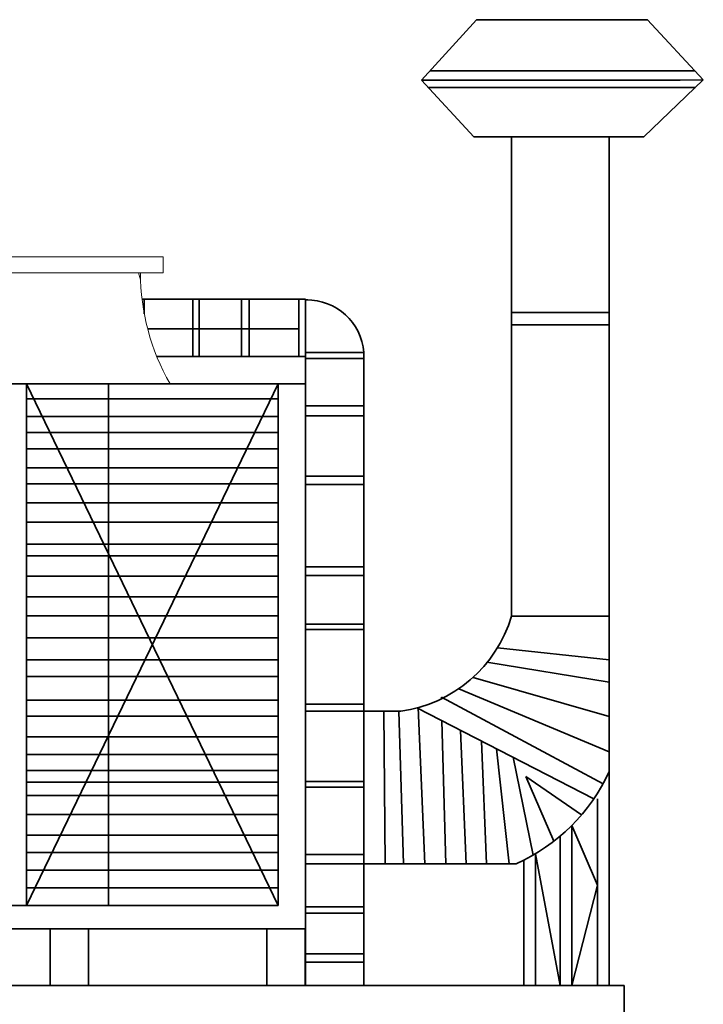
# Model space of a CAD drawing. Units: inches. Extents: x -1080 to 1950, y -1929 to 857.
# Tile 11 of 16: x 1333 to 1474, y -633 to -430. Entities that reach past the tile are written whole.
import ezdxf

# ---------------------------------------------------------------- set-up
doc = ezdxf.new("R2010")
doc.units = ezdxf.units.IN
doc.header["$MEASUREMENT"] = 0
doc.layers.add('A-DOOR', color=3, linetype='Continuous', lineweight=18)
doc.layers.add('A-ELEV', color=7, linetype='Continuous', lineweight=35)

# ---------------------------------------------------------------- blocks, each defined once
blk = doc.blocks.new('DOOR-DOUBLE')
for p, q in [((0.57, 22.87), (0.57, 26.22)), ((0.57, 26.22), (41.91, 26.22)), ((41.91, 26.22), (41.91, 22.87)), ((5.34, 22.87), (0.57, 22.87)), ((5.34, 22.87), (37.21, 22.87)), ((36.82, 22.87), (37.23, 21.43)), ((41.91, 22.87), (37.21, 22.87)), ((0, 0), (43.32, 0))]:
    blk.add_line(p, q)
for centre, radius, start, end in [((-50.66, 22.94), 55.61, 335.64, 359.9307), ((83.27, 22.93), 46.06, 180.0717, 209.8526)]:
    blk.add_arc(centre, radius, start, end)

msp = doc.modelspace()

# ---------------------------------------------------------------- linework, layer by layer
at = {"layer": 'A-ELEV'}
for p, q in [((1427.51, -430.18), (1416.21, -442.66)), ((1427.51, -430.18), (1462.88, -430.18)), ((1462.88, -430.18), (1474.38, -442.61)), ((1417.95, -440.74), (1470.17, -440.74)), ((1470.17, -440.74), (1472.63, -440.72)), ((1426.96, -454.38), (1416.21, -442.66)), ((1416.21, -442.66), (1469.6, -442.66)), ((1462.11, -454.38), (1474.38, -442.61)), ((1469.6, -442.66), (1474.38, -442.61)), ((1417.62, -444.2), (1470.17, -444.2)), ((1470.17, -444.2), (1472.76, -444.17)), ((1426.96, -454.38), (1462.11, -454.38)), ((1426.96, -454.38), (1462.11, -454.38)), ((1434.79, -553.32), (1434.79, -454.49)), ((1454.95, -585.43), (1454.95, -454.49)), ((1358.46, -487.89), (1392.19, -487.89)), ((1358.91, -490.88), (1358.91, -487.89)), ((1368.96, -499.75), (1368.96, -487.89)), ((1370.29, -499.75), (1370.29, -487.89)), ((1379.03, -499.75), (1379.03, -487.89)), ((1380.6, -499.75), (1380.6, -487.89)), ((1390.84, -499.75), (1390.84, -487.89)), ((1392.19, -487.89), (1392.19, -629.59)), ((1392.38, -488.03), (1392.71, -488.03)), ((1434.79, -490.63), (1454.95, -490.63)), ((1359.61, -493.99), (1390.84, -493.99)), ((1434.79, -493.16), (1454.95, -493.16)), ((1361.52, -499.75), (1392.19, -499.75)), ((1392.18, -498.89), (1404.26, -498.89)), ((1404.26, -498.89), (1404.26, -629.59)), ((1392.18, -500.17), (1404.26, -500.17)), ((1179.83, -505.38), (1392.19, -505.38)), ((1334.58, -613.11), (1334.58, -505.38)), ((1334.58, -505.38), (1386.54, -613.11)), ((1386.54, -505.38), (1334.58, -613.11)), ((1334.58, -505.38), (1386.54, -505.38)), ((1351.51, -613.11), (1351.51, -505.38)), ((1386.54, -505.38), (1386.54, -613.11)), ((1386.54, -613.11), (1386.54, -505.38)), ((1334.58, -508.47), (1386.54, -508.47)), ((1392.18, -509.89), (1404.26, -509.89)), ((1334.58, -512.1), (1386.54, -512.1)), ((1392.18, -511.94), (1404.26, -511.94)), ((1334.58, -515.43), (1386.54, -515.43)), ((1334.58, -518.77), (1386.54, -518.77)), ((1334.58, -522.7), (1386.54, -522.7)), ((1392.18, -524.4), (1404.26, -524.4)), ((1334.58, -526.03), (1386.54, -526.03)), ((1392.18, -526.16), (1404.26, -526.16)), ((1392.18, -527.19), (1392.19, -527.19)), ((1392.18, -527.19), (1392.19, -527.19)), ((1334.58, -529.97), (1386.54, -529.97)), ((1334.58, -533.91), (1386.54, -533.91)), ((1334.58, -538.45), (1386.54, -538.45)), ((1334.58, -540.87), (1386.54, -540.87)), ((1392.18, -543.15), (1404.26, -543.15)), ((1334.58, -545.11), (1386.54, -545.11)), ((1392.18, -544.91), (1404.26, -544.91)), ((1334.58, -549.35), (1386.54, -549.35)), ((1334.58, -553.29), (1386.54, -553.29)), ((1434.79, -553.32), (1454.95, -553.32)), ((1392.18, -555.02), (1404.26, -555.02)), ((1392.18, -556.06), (1404.26, -556.06)), ((1334.58, -557.83), (1386.54, -557.83)), ((1454.95, -562.36), (1431.86, -559.89)), ((1334.58, -562.37), (1386.54, -562.37)), ((1454.95, -566.97), (1429.67, -562.81)), ((1429.69, -562.96), (1429.67, -562.81)), ((1334.58, -565.82), (1386.54, -565.82)), ((1454.95, -574.04), (1426.84, -565.97)), ((1454.95, -581.34), (1423.88, -568.31)), ((1423.88, -568.31), (1423.88, -568.31)), ((1334.58, -570.67), (1386.54, -570.67)), ((1453.68, -587.94), (1420.29, -570.08)), ((1420.29, -570.41), (1420.29, -570.08)), ((1392.18, -571.53), (1404.26, -571.53)), ((1392.18, -572.97), (1404.26, -572.97)), ((1404.26, -572.97), (1411.88, -572.97)), ((1408.64, -604.46), (1408.42, -572.97)), ((1412.43, -604.46), (1411.51, -572.97)), ((1451.78, -591.03), (1415.21, -572.3)), ((1416.89, -604.46), (1415.5, -572.22)), ((1334.58, -574), (1386.54, -574)), ((1421.17, -604.46), (1420.41, -574.97)), ((1425.43, -604.46), (1424.25, -576.93)), ((1334.58, -578.24), (1386.54, -578.24)), ((1429.63, -604.46), (1428.54, -579.13)), ((1434.3, -604.46), (1431.66, -580.73)), ((1334.58, -581.87), (1386.54, -581.87)), ((1439.24, -602.67), (1435.09, -582.48)), ((1334.58, -585.21), (1386.54, -585.21)), ((1454.95, -585.43), (1454.95, -629.59)), ((1392.18, -587.48), (1404.26, -587.48)), ((1449.23, -594.36), (1437.71, -586.47)), ((1443.53, -599.8), (1437.71, -586.47)), ((1334.58, -587.63), (1386.54, -587.63)), ((1392.18, -588.68), (1404.26, -588.68)), ((1334.58, -590.35), (1386.54, -590.35)), ((1452.52, -629.59), (1452.52, -591.03)), ((1334.58, -594.29), (1386.54, -594.29)), ((1447.24, -596.53), (1447.24, -629.59)), ((1452.52, -608.85), (1447.24, -596.53)), ((1334.58, -598.53), (1386.54, -598.53)), ((1444.81, -629.59), (1444.81, -598.76)), ((1334.58, -602.16), (1386.54, -602.16)), ((1392.18, -602.54), (1404.26, -602.54)), ((1437.32, -629.59), (1437.32, -603.71)), ((1439.74, -602.38), (1439.74, -629.59)), ((1439.74, -602.38), (1444.81, -629.59)), ((1334.58, -605.8), (1386.54, -605.8)), ((1392.18, -604.46), (1404.26, -604.46)), ((1404.26, -604.46), (1435.75, -604.46)), ((1334.58, -609.43), (1386.54, -609.43)), ((1447.24, -629.59), (1452.52, -608.85)), ((1386.54, -613.11), (1183.24, -613.11)), ((1392.18, -613.36), (1404.26, -613.36)), ((1392.18, -614.64), (1404.26, -614.64)), ((1179.83, -617.91), (1392.19, -617.91)), ((1339.47, -617.91), (1339.47, -629.59)), ((1347.4, -617.91), (1347.4, -629.59)), ((1384.25, -617.91), (1384.25, -629.59)), ((1392.18, -617.91), (1392.18, -629.59)), ((1392.18, -623.04), (1404.26, -623.04)), ((1392.18, -624.8), (1404.26, -624.8)), ((1458.07, -629.59), (1120.45, -629.59)), ((1458.07, -680.68), (1458.07, -629.59))]:
    msp.add_line(p, q, dxfattribs=at)
for centre, radius, start, end in [((1392.54, -499.78), 11.75, 4.3338, 90.8097), ((1408.07, -545.35), 27.88, 277.8523, 343.3919), ((1420.01, -569.38), 38.45, 294.1679, 335.322)]:
    msp.add_arc(centre, radius, start, end, dxfattribs=at)

# ---------------------------------------------------------------- block references
at = {"layer": 'A-DOOR'}
msp.add_blockref('DOOR-DOUBLE', (1320.92, -505.35), dxfattribs=at)

doc.saveas('drawing.dxf')
